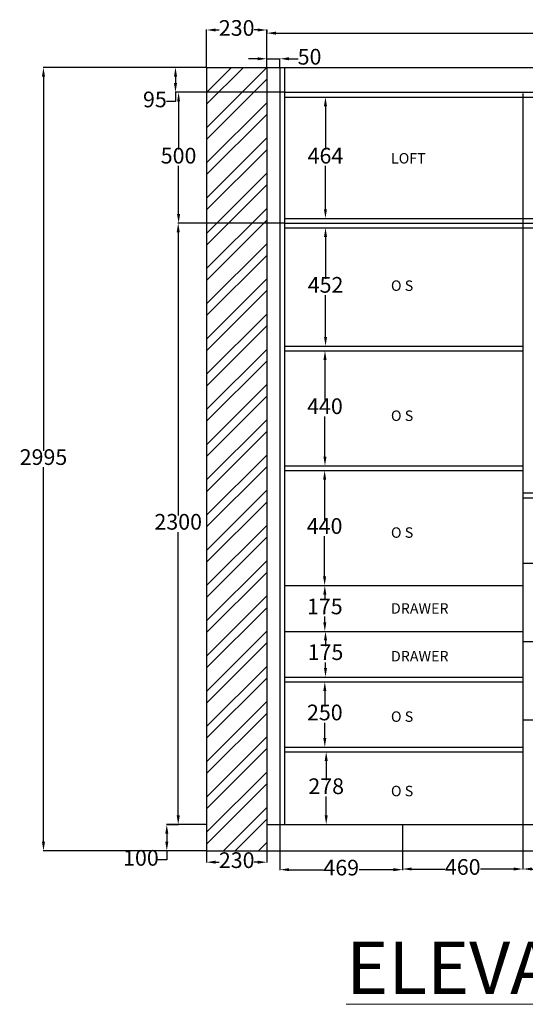
# Model space of a CAD drawing. Units: millimetres. Extents: x 1304 to 14372, y 283 to 7516.
# Tile 1 of 4: x 1304 to 3237, y 283 to 4048. Entities that reach past the tile are written whole.
import ezdxf

# ---------------------------------------------------------------- set-up
doc = ezdxf.new("R2010")
doc.units = ezdxf.units.MM
doc.layers.get('Defpoints').update_dxf_attribs({"color": 2})
for name, color, linetype, lineweight in [('A-ANNO-DIMS', 2, 'Continuous', 18), ('A-ANNO-TEXT', 3, 'Continuous', 18), ('A-FURN', 7, 'Continuous', 25), ('A-FURN-PATT', 8, 'Continuous', 13)]:
    doc.layers.add(name, color=color, linetype=linetype, lineweight=lineweight)
doc.styles.get("Standard").update_dxf_attribs({"font": 'arial.ttf'})
doc.dimstyles.new('ISO-25', dxfattribs={"dimtxt": 60, "dimasz": 35, "dimexe": 1.25, "dimexo": 0.625, "dimtad": 0, "dimtih": 1, "dimtoh": 1, "dimtxsty": 'Standard', "dimcen": 2.5, "dimclrd": 1, "dimclre": 3, "dimadec": 0, "dimazin": 0, "dimtfac": 1, "dimtmove": 0, "dimatfit": 3, "dimfxl": 1, "dimarcsym": 0})

# ---------------------------------------------------------------- blocks, each defined once
blk = doc.blocks.new('*D1')
at = {"layer": 'A-ANNO-DIMS', "color": 0, "lineweight": -2, "transparency": 16777216}
for p, q in [((2317.3, 3752.3), (2474.1, 3752.3)), ((2472.8, 3717.3), (2472.8, 3551.5)), ((2472.8, 3323.3), (2472.8, 3489)), ((2317.3, 3288.3), (2474.1, 3288.3))]:
    blk.add_line(p, q, dxfattribs=at)
at = {"layer": 'A-ANNO-DIMS', "color": 0, "transparency": 16777216}
for points in [[(2467, 3717.3), (2478.7, 3717.3), (2472.8, 3752.3)], [(2467, 3323.3), (2478.7, 3323.3), (2472.8, 3288.3)]]:
    blk.add_solid(points, dxfattribs=at)
at = {"layer": 'Defpoints', "color": 0, "transparency": 16777216}
for p in [(2316.6, 3752.3), (2316.6, 3288.3), (2472.8, 3288.3)]:
    blk.add_point(p, dxfattribs=at)
at = {"layer": 'A-ANNO-DIMS', "color": 0, "transparency": 16777216, "insert": (2472.8, 3520.3), "char_height": 60, "attachment_point": 5}
blk.add_mtext('464', dxfattribs=at)
blk = doc.blocks.new('*D2')
at = {"layer": 'A-ANNO-DIMS', "color": 0, "lineweight": -2, "transparency": 16777216}
for p, q in [((2317.3, 3252.3), (2474.4, 3252.3)), ((2473.2, 3217.3), (2473.2, 3057.5)), ((2473.2, 2835.3), (2473.2, 2995)), ((2317.3, 2800.3), (2474.4, 2800.3))]:
    blk.add_line(p, q, dxfattribs=at)
at = {"layer": 'A-ANNO-DIMS', "color": 0, "transparency": 16777216}
for points in [[(2467.4, 3217.3), (2479, 3217.3), (2473.2, 3252.3)], [(2467.4, 2835.3), (2479, 2835.3), (2473.2, 2800.3)]]:
    blk.add_solid(points, dxfattribs=at)
at = {"layer": 'Defpoints', "color": 0, "transparency": 16777216}
for p in [(2316.6, 3252.3), (2316.6, 2800.3), (2473.2, 2800.3)]:
    blk.add_point(p, dxfattribs=at)
at = {"layer": 'A-ANNO-DIMS', "color": 0, "transparency": 16777216, "insert": (2473.2, 3026.3), "char_height": 60, "attachment_point": 5}
blk.add_mtext('452', dxfattribs=at)
blk = doc.blocks.new('*D3')
at = {"layer": 'A-ANNO-DIMS', "color": 0, "lineweight": -2, "transparency": 16777216}
for p, q in [((2317.3, 2782.3), (2472.3, 2782.3)), ((2471, 2747.3), (2471, 2593.5)), ((2471, 2377.3), (2471, 2531)), ((2317.3, 2342.3), (2472.3, 2342.3))]:
    blk.add_line(p, q, dxfattribs=at)
at = {"layer": 'A-ANNO-DIMS', "color": 0, "transparency": 16777216}
for points in [[(2465.2, 2747.3), (2476.9, 2747.3), (2471, 2782.3)], [(2465.2, 2377.3), (2476.9, 2377.3), (2471, 2342.3)]]:
    blk.add_solid(points, dxfattribs=at)
at = {"layer": 'Defpoints', "color": 0, "transparency": 16777216}
for p in [(2316.6, 2782.3), (2316.6, 2342.3), (2471, 2342.3)]:
    blk.add_point(p, dxfattribs=at)
at = {"layer": 'A-ANNO-DIMS', "color": 0, "transparency": 16777216, "insert": (2471, 2562.3), "char_height": 60, "attachment_point": 5}
blk.add_mtext('440', dxfattribs=at)
blk = doc.blocks.new('*D4')
at = {"layer": 'A-ANNO-DIMS', "color": 0, "lineweight": -2, "transparency": 16777216}
for p, q in [((2317.3, 2324.3), (2470.9, 2324.3)), ((2469.7, 2289.3), (2469.7, 2135.5)), ((2469.7, 1919.3), (2469.7, 2073)), ((2317.3, 1884.3), (2470.9, 1884.3))]:
    blk.add_line(p, q, dxfattribs=at)
at = {"layer": 'A-ANNO-DIMS', "color": 0, "transparency": 16777216}
for points in [[(2463.8, 2289.3), (2475.5, 2289.3), (2469.7, 2324.3)], [(2463.8, 1919.3), (2475.5, 1919.3), (2469.7, 1884.3)]]:
    blk.add_solid(points, dxfattribs=at)
at = {"layer": 'Defpoints', "color": 0, "transparency": 16777216}
for p in [(2316.6, 2324.3), (2316.6, 1884.3), (2469.7, 1884.3)]:
    blk.add_point(p, dxfattribs=at)
at = {"layer": 'A-ANNO-DIMS', "color": 0, "transparency": 16777216, "insert": (2469.7, 2104.3), "char_height": 60, "attachment_point": 5}
blk.add_mtext('440', dxfattribs=at)
blk = doc.blocks.new('*D5')
at = {"layer": 'A-ANNO-DIMS', "color": 0, "lineweight": -2, "transparency": 16777216}
for p, q in [((2317.3, 1884.3), (2471.6, 1884.3)), ((2470.4, 1849.3), (2470.4, 1828)), ((2470.4, 1744.3), (2470.4, 1765.5)), ((2317.3, 1709.3), (2471.6, 1709.3))]:
    blk.add_line(p, q, dxfattribs=at)
at = {"layer": 'A-ANNO-DIMS', "color": 0, "transparency": 16777216}
for points in [[(2464.5, 1849.3), (2476.2, 1849.3), (2470.4, 1884.3)], [(2464.5, 1744.3), (2476.2, 1744.3), (2470.4, 1709.3)]]:
    blk.add_solid(points, dxfattribs=at)
at = {"layer": 'Defpoints', "color": 0, "transparency": 16777216}
for p in [(2316.6, 1884.3), (2316.6, 1709.3), (2470.4, 1709.3)]:
    blk.add_point(p, dxfattribs=at)
at = {"layer": 'A-ANNO-DIMS', "color": 0, "transparency": 16777216, "insert": (2470.4, 1796.8), "char_height": 60, "attachment_point": 5}
blk.add_mtext('175', dxfattribs=at)
blk = doc.blocks.new('*D6')
at = {"layer": 'A-ANNO-DIMS', "color": 0, "lineweight": -2, "transparency": 16777216}
for p, q in [((2317.3, 1709.3), (2474.3, 1709.3)), ((2473, 1674.3), (2473, 1653)), ((2473, 1569.3), (2473, 1590.5)), ((2317.3, 1534.3), (2474.3, 1534.3))]:
    blk.add_line(p, q, dxfattribs=at)
at = {"layer": 'A-ANNO-DIMS', "color": 0, "transparency": 16777216}
for points in [[(2467.2, 1674.3), (2478.8, 1674.3), (2473, 1709.3)], [(2467.2, 1569.3), (2478.8, 1569.3), (2473, 1534.3)]]:
    blk.add_solid(points, dxfattribs=at)
at = {"layer": 'Defpoints', "color": 0, "transparency": 16777216}
for p in [(2316.6, 1709.3), (2316.6, 1534.3), (2473, 1534.3)]:
    blk.add_point(p, dxfattribs=at)
at = {"layer": 'A-ANNO-DIMS', "color": 0, "transparency": 16777216, "insert": (2473, 1621.8), "char_height": 60, "attachment_point": 5}
blk.add_mtext('175', dxfattribs=at)
blk = doc.blocks.new('*D7')
at = {"layer": 'A-ANNO-DIMS', "color": 0, "lineweight": -2, "transparency": 16777216}
for p, q in [((2317.3, 1516.3), (2471.6, 1516.3)), ((2470.4, 1481.3), (2470.4, 1422.5)), ((2470.4, 1301.3), (2470.4, 1360)), ((2317.3, 1266.3), (2471.6, 1266.3))]:
    blk.add_line(p, q, dxfattribs=at)
at = {"layer": 'A-ANNO-DIMS', "color": 0, "transparency": 16777216}
for points in [[(2464.5, 1481.3), (2476.2, 1481.3), (2470.4, 1516.3)], [(2464.5, 1301.3), (2476.2, 1301.3), (2470.4, 1266.3)]]:
    blk.add_solid(points, dxfattribs=at)
at = {"layer": 'Defpoints', "color": 0, "transparency": 16777216}
for p in [(2316.6, 1516.3), (2316.6, 1266.3), (2470.4, 1266.3)]:
    blk.add_point(p, dxfattribs=at)
at = {"layer": 'A-ANNO-DIMS', "color": 0, "transparency": 16777216, "insert": (2470.4, 1391.3), "char_height": 60, "attachment_point": 5}
blk.add_mtext('250', dxfattribs=at)
blk = doc.blocks.new('*D8')
at = {"layer": 'A-ANNO-DIMS', "color": 0, "lineweight": -2, "transparency": 16777216}
for p, q in [((2317.3, 1248.3), (2476.9, 1248.3)), ((2475.7, 1213.3), (2475.7, 1140.5)), ((2475.7, 1005.3), (2475.7, 1078)), ((2317.3, 970.3), (2476.9, 970.3))]:
    blk.add_line(p, q, dxfattribs=at)
at = {"layer": 'A-ANNO-DIMS', "color": 0, "transparency": 16777216}
for points in [[(2469.8, 1213.3), (2481.5, 1213.3), (2475.7, 1248.3)], [(2469.8, 1005.3), (2481.5, 1005.3), (2475.7, 970.3)]]:
    blk.add_solid(points, dxfattribs=at)
at = {"layer": 'Defpoints', "color": 0, "transparency": 16777216}
for p in [(2316.6, 1248.3), (2316.6, 970.3), (2475.7, 970.3)]:
    blk.add_point(p, dxfattribs=at)
at = {"layer": 'A-ANNO-DIMS', "color": 0, "transparency": 16777216, "insert": (2475.7, 1109.3), "char_height": 60, "attachment_point": 5}
blk.add_mtext('278', dxfattribs=at)
blk = doc.blocks.new('*D9')
at = {"layer": 'A-ANNO-DIMS', "color": 0, "lineweight": -2, "transparency": 16777216}
for p, q in [((2018, 3865.3), (1393.8, 3865.3)), ((1395.1, 3830.3), (1395.1, 2399)), ((1395.1, 905.3), (1395.1, 2336.5)), ((2018, 870.3), (1393.8, 870.3))]:
    blk.add_line(p, q, dxfattribs=at)
at = {"layer": 'A-ANNO-DIMS', "color": 0, "transparency": 16777216}
for points in [[(1389.3, 3830.3), (1400.9, 3830.3), (1395.1, 3865.3)], [(1389.3, 905.3), (1400.9, 905.3), (1395.1, 870.3)]]:
    blk.add_solid(points, dxfattribs=at)
at = {"layer": 'Defpoints', "color": 0, "transparency": 16777216}
for p in [(2018.6, 3865.3), (1395.1, 870.3), (2018.6, 870.3)]:
    blk.add_point(p, dxfattribs=at)
at = {"layer": 'A-ANNO-DIMS', "color": 0, "transparency": 16777216, "insert": (1395.1, 2367.8), "char_height": 60, "attachment_point": 5}
blk.add_mtext('2995', dxfattribs=at)
blk = doc.blocks.new('*D10')
at = {"layer": 'A-ANNO-DIMS', "color": 0, "lineweight": -2, "transparency": 16777216}
for p, q in [((2018, 3865.3), (1898.5, 3865.3)), ((1899.7, 3830.3), (1899.7, 3805.3)), ((2018, 3770.3), (1898.5, 3770.3)), ((1899.7, 3770.3), (1899.7, 3735.3)), ((1899.7, 3735.3), (1864.7, 3735.3))]:
    blk.add_line(p, q, dxfattribs=at)
at = {"layer": 'A-ANNO-DIMS', "color": 0, "transparency": 16777216}
for points in [[(1893.9, 3830.3), (1905.6, 3830.3), (1899.7, 3865.3)], [(1893.9, 3805.3), (1905.6, 3805.3), (1899.7, 3770.3)]]:
    blk.add_solid(points, dxfattribs=at)
at = {"layer": 'Defpoints', "color": 0, "transparency": 16777216}
for p in [(2018.6, 3865.3), (1899.7, 3770.3), (2018.6, 3770.3)]:
    blk.add_point(p, dxfattribs=at)
at = {"layer": 'A-ANNO-DIMS', "color": 0, "transparency": 16777216, "insert": (1820.9, 3735.3), "char_height": 60, "attachment_point": 5}
blk.add_mtext('95', dxfattribs=at)
blk = doc.blocks.new('*D11')
at = {"layer": 'A-ANNO-DIMS', "color": 0, "lineweight": -2, "transparency": 16777216}
for p, q in [((2316, 3770.3), (1910.2, 3770.3)), ((1911.5, 3735.3), (1911.5, 3551.5)), ((1911.5, 3305.3), (1911.5, 3489)), ((2316, 3270.3), (1910.2, 3270.3))]:
    blk.add_line(p, q, dxfattribs=at)
at = {"layer": 'A-ANNO-DIMS', "color": 0, "transparency": 16777216}
for points in [[(1905.7, 3735.3), (1917.3, 3735.3), (1911.5, 3770.3)], [(1905.7, 3305.3), (1917.3, 3305.3), (1911.5, 3270.3)]]:
    blk.add_solid(points, dxfattribs=at)
at = {"layer": 'Defpoints', "color": 0, "transparency": 16777216}
for p in [(2316.6, 3770.3), (1911.5, 3270.3), (2316.6, 3270.3)]:
    blk.add_point(p, dxfattribs=at)
at = {"layer": 'A-ANNO-DIMS', "color": 0, "transparency": 16777216, "insert": (1911.5, 3520.3), "char_height": 60, "attachment_point": 5}
blk.add_mtext('500', dxfattribs=at)
blk = doc.blocks.new('*D12')
at = {"layer": 'A-ANNO-DIMS', "color": 0, "lineweight": -2, "transparency": 16777216}
for p, q in [((2018, 970.3), (1865.2, 970.3)), ((1866.4, 935.3), (1866.4, 905.3)), ((2018, 870.3), (1865.2, 870.3)), ((1866.4, 870.3), (1866.4, 835.3)), ((1866.4, 835.3), (1831.4, 835.3))]:
    blk.add_line(p, q, dxfattribs=at)
at = {"layer": 'A-ANNO-DIMS', "color": 0, "transparency": 16777216}
for points in [[(1860.6, 935.3), (1872.3, 935.3), (1866.4, 970.3)], [(1860.6, 905.3), (1872.3, 905.3), (1866.4, 870.3)]]:
    blk.add_solid(points, dxfattribs=at)
at = {"layer": 'Defpoints', "color": 0, "transparency": 16777216}
for p in [(2018.6, 970.3), (1866.4, 870.3), (2018.6, 870.3)]:
    blk.add_point(p, dxfattribs=at)
at = {"layer": 'A-ANNO-DIMS', "color": 0, "transparency": 16777216, "insert": (1767.5, 835.3), "char_height": 60, "attachment_point": 5}
blk.add_mtext('100', dxfattribs=at)
blk = doc.blocks.new('*D13')
at = {"layer": 'A-ANNO-DIMS', "color": 0, "lineweight": -2, "transparency": 16777216}
for p, q in [((1910.9, 3270.3), (1908.9, 3270.3)), ((1910.1, 3235.3), (1910.1, 2151.6)), ((1910.1, 1005.3), (1910.1, 2089)), ((1867.1, 970.3), (1911.4, 970.3))]:
    blk.add_line(p, q, dxfattribs=at)
at = {"layer": 'A-ANNO-DIMS', "color": 0, "transparency": 16777216}
for points in [[(1904.3, 3235.3), (1916, 3235.3), (1910.1, 3270.3)], [(1904.3, 1005.3), (1916, 1005.3), (1910.1, 970.3)]]:
    blk.add_solid(points, dxfattribs=at)
at = {"layer": 'Defpoints', "color": 0, "transparency": 16777216}
for p in [(1910.1, 3270.3), (1911.5, 3270.3), (1866.4, 970.3)]:
    blk.add_point(p, dxfattribs=at)
at = {"layer": 'A-ANNO-DIMS', "color": 0, "transparency": 16777216, "insert": (1910.1, 2120.3), "char_height": 60, "attachment_point": 5}
blk.add_mtext('2300', dxfattribs=at)
blk = doc.blocks.new('*D14')
at = {"layer": 'A-ANNO-DIMS', "color": 0, "lineweight": -2, "transparency": 16777216}
for p, q in [((2213.6, 3898.5), (2178.6, 3898.5)), ((2248.6, 3865.9), (2248.6, 3899.8)), ((2248.6, 3898.5), (2298.6, 3898.5)), ((2298.6, 3865.9), (2298.6, 3899.8)), ((2333.6, 3898.5), (2368.6, 3898.5))]:
    blk.add_line(p, q, dxfattribs=at)
at = {"layer": 'A-ANNO-DIMS', "color": 0, "transparency": 16777216}
for points in [[(2213.6, 3904.4), (2213.6, 3892.7), (2248.6, 3898.5)], [(2333.6, 3904.4), (2333.6, 3892.7), (2298.6, 3898.5)]]:
    blk.add_solid(points, dxfattribs=at)
at = {"layer": 'Defpoints', "color": 0, "transparency": 16777216}
for p in [(2298.6, 3898.5), (2248.6, 3865.3), (2298.6, 3865.3)]:
    blk.add_point(p, dxfattribs=at)
at = {"layer": 'A-ANNO-DIMS', "color": 0, "transparency": 16777216, "insert": (2412.1, 3898.5), "char_height": 60, "attachment_point": 5}
blk.add_mtext('50', dxfattribs=at)
blk = doc.blocks.new('*D15')
at = {"layer": 'A-ANNO-DIMS', "color": 0, "lineweight": -2, "transparency": 16777216}
for p, q in [((2018.6, 3865.9), (2018.6, 4009.9)), ((2053.6, 4008.6), (2066.3, 4008.6)), ((2213.6, 4008.6), (2201, 4008.6)), ((2248.6, 3865.9), (2248.6, 4009.9))]:
    blk.add_line(p, q, dxfattribs=at)
at = {"layer": 'A-ANNO-DIMS', "color": 0, "transparency": 16777216}
for points in [[(2053.6, 4014.4), (2053.6, 4002.8), (2018.6, 4008.6)], [(2213.6, 4014.4), (2213.6, 4002.8), (2248.6, 4008.6)]]:
    blk.add_solid(points, dxfattribs=at)
at = {"layer": 'Defpoints', "color": 0, "transparency": 16777216}
for p in [(2248.6, 4008.6), (2018.6, 3865.3), (2248.6, 3865.3)]:
    blk.add_point(p, dxfattribs=at)
at = {"layer": 'A-ANNO-DIMS', "color": 0, "transparency": 16777216, "insert": (2133.6, 4008.6), "char_height": 60, "attachment_point": 5}
blk.add_mtext('230', dxfattribs=at)
blk = doc.blocks.new('*D16')
at = {"layer": 'A-ANNO-DIMS', "color": 0, "lineweight": -2, "transparency": 16777216}
for p, q in [((2248.6, 4008), (2248.6, 3995.4)), ((2283.6, 3996.6), (4728.5, 3996.6)), ((7353.6, 3996.6), (4908.8, 3996.6)), ((7388.6, 3865.9), (7388.6, 3997.9))]:
    blk.add_line(p, q, dxfattribs=at)
at = {"layer": 'A-ANNO-DIMS', "color": 0, "transparency": 16777216}
for points in [[(2283.6, 4002.4), (2283.6, 3990.8), (2248.6, 3996.6)], [(7353.6, 4002.4), (7353.6, 3990.8), (7388.6, 3996.6)]]:
    blk.add_solid(points, dxfattribs=at)
at = {"layer": 'Defpoints', "color": 0, "transparency": 16777216}
for p in [(2248.6, 4008.6), (7388.6, 3996.6), (7388.6, 3865.3)]:
    blk.add_point(p, dxfattribs=at)
at = {"layer": 'A-ANNO-DIMS', "color": 0, "transparency": 16777216, "insert": (4818.6, 3996.6), "char_height": 60, "attachment_point": 5}
blk.add_mtext('5140', dxfattribs=at)
blk = doc.blocks.new('*D33')
at = {"layer": 'A-ANNO-DIMS', "color": 0, "lineweight": -2, "transparency": 16777216}
for p, q in [((2018.6, 869.7), (2018.6, 825.4)), ((2248.6, 869.7), (2248.6, 825.4)), ((2053.6, 826.6), (2066.3, 826.6)), ((2213.6, 826.6), (2201, 826.6))]:
    blk.add_line(p, q, dxfattribs=at)
at = {"layer": 'A-ANNO-DIMS', "color": 0, "transparency": 16777216}
for points in [[(2053.6, 832.4), (2053.6, 820.8), (2018.6, 826.6)], [(2213.6, 832.4), (2213.6, 820.8), (2248.6, 826.6)]]:
    blk.add_solid(points, dxfattribs=at)
at = {"layer": 'Defpoints', "color": 0, "transparency": 16777216}
for p in [(2018.6, 870.3), (2248.6, 870.3), (2248.6, 826.6)]:
    blk.add_point(p, dxfattribs=at)
at = {"layer": 'A-ANNO-DIMS', "color": 0, "transparency": 16777216, "insert": (2133.6, 826.6), "char_height": 60, "attachment_point": 5}
blk.add_mtext('230', dxfattribs=at)
blk = doc.blocks.new('*D34')
at = {"layer": 'A-ANNO-DIMS', "color": 0, "lineweight": -2, "transparency": 16777216}
for p, q in [((2298.6, 969.7), (2298.6, 796.7)), ((2767.6, 863.2), (2767.6, 796.7)), ((2333.6, 798), (2465, 798)), ((2732.6, 798), (2601.3, 798))]:
    blk.add_line(p, q, dxfattribs=at)
at = {"layer": 'A-ANNO-DIMS', "color": 0, "transparency": 16777216}
for points in [[(2333.6, 803.8), (2333.6, 792.2), (2298.6, 798)], [(2732.6, 803.8), (2732.6, 792.2), (2767.6, 798)]]:
    blk.add_solid(points, dxfattribs=at)
at = {"layer": 'Defpoints', "color": 0, "transparency": 16777216}
for p in [(2298.6, 970.3), (2767.6, 863.8), (2767.6, 798)]:
    blk.add_point(p, dxfattribs=at)
at = {"layer": 'A-ANNO-DIMS', "color": 0, "transparency": 16777216, "insert": (2533.1, 798), "char_height": 60, "attachment_point": 5}
blk.add_mtext('469', dxfattribs=at)
blk = doc.blocks.new('*D35')
at = {"layer": 'A-ANNO-DIMS', "color": 0, "lineweight": -2, "transparency": 16777216}
for p, q in [((2767.6, 969.7), (2767.6, 799.2)), ((3227.6, 969.7), (3227.6, 799.2)), ((2802.6, 800.5), (2929.6, 800.5)), ((3192.6, 800.5), (3065.7, 800.5))]:
    blk.add_line(p, q, dxfattribs=at)
at = {"layer": 'A-ANNO-DIMS', "color": 0, "transparency": 16777216}
for points in [[(2802.6, 806.3), (2802.6, 794.7), (2767.6, 800.5)], [(3192.6, 806.3), (3192.6, 794.7), (3227.6, 800.5)]]:
    blk.add_solid(points, dxfattribs=at)
at = {"layer": 'Defpoints', "color": 0, "transparency": 16777216}
for p in [(2767.6, 970.3), (3227.6, 970.3), (3227.6, 800.5)]:
    blk.add_point(p, dxfattribs=at)
at = {"layer": 'A-ANNO-DIMS', "color": 0, "transparency": 16777216, "insert": (2997.6, 800.5), "char_height": 60, "attachment_point": 5}
blk.add_mtext('460', dxfattribs=at)
blk = doc.blocks.new('*D36')
at = {"layer": 'A-ANNO-DIMS', "color": 0, "lineweight": -2, "transparency": 16777216}
for p, q in [((3227.6, 801.1), (3227.6, 801.7)), ((3262.6, 800.5), (3389.6, 800.5)), ((3652.6, 800.5), (3525.7, 800.5)), ((3687.6, 801.1), (3687.6, 801.7))]:
    blk.add_line(p, q, dxfattribs=at)
at = {"layer": 'A-ANNO-DIMS', "color": 0, "transparency": 16777216}
for points in [[(3262.6, 806.3), (3262.6, 794.7), (3227.6, 800.5)], [(3652.6, 806.3), (3652.6, 794.7), (3687.6, 800.5)]]:
    blk.add_solid(points, dxfattribs=at)
at = {"layer": 'Defpoints', "color": 0, "transparency": 16777216}
for p in [(3227.6, 800.5), (3687.6, 800.5), (3687.6, 800.5)]:
    blk.add_point(p, dxfattribs=at)
at = {"layer": 'A-ANNO-DIMS', "color": 0, "transparency": 16777216, "insert": (3457.6, 800.5), "char_height": 60, "attachment_point": 5}
blk.add_mtext('460', dxfattribs=at)

msp = doc.modelspace()

# ---------------------------------------------------------------- hatches: boundary and pattern name
at = {"layer": 'A-FURN-PATT'}
h = msp.add_hatch(dxfattribs=at)
h.set_pattern_fill('ANSI32', color=256, scale=10)
h.paths.add_polyline_path([(2018.643, 870.285), (2248.643, 870.285), (2248.643, 3865.285), (2018.643, 3865.285)])
h.paths.add_polyline_path([(7388.643, 870.285), (7618.643, 870.285), (7618.643, 3865.285), (7388.643, 3865.285)])

# ---------------------------------------------------------------- linework, layer by layer
at = {"layer": 'A-FURN'}
for p, q in [((2018.643, 3865.285), (2018.643, 870.285)), ((2018.643, 3865.285), (7618.643, 3865.285)), ((2248.643, 3865.285), (2248.643, 870.285)), ((2298.643, 3865.285), (2298.643, 970.285)), ((2316.643, 3865.285), (2316.643, 970.285)), ((2316.643, 3770.285), (7388.643, 3770.285)), ((3227.643, 3765.285), (3227.643, 970.285)), ((2316.643, 3752.285), (5067.643, 3752.285)), ((2316.643, 3288.285), (5067.643, 3288.285)), ((2316.643, 3270.285), (5545.643, 3270.285)), ((2316.643, 3252.285), (4165.643, 3252.285)), ((2316.643, 2800.285), (3227.643, 2800.285)), ((2316.643, 2782.285), (3227.643, 2782.285)), ((2316.643, 2342.285), (3227.643, 2342.285)), ((2316.643, 2324.285), (3227.643, 2324.285)), ((3227.643, 2238.285), (4147.643, 2238.285)), ((3227.643, 2220.285), (4147.643, 2220.285)), ((3227.643, 1970.285), (4147.643, 1970.285)), ((2316.643, 1884.285), (3227.643, 1884.285)), ((2316.643, 1709.285), (3227.643, 1709.285)), ((3227.643, 1670.285), (4147.643, 1670.285)), ((2316.643, 1534.285), (3227.643, 1534.285)), ((2316.643, 1516.285), (3227.643, 1516.285)), ((3227.643, 1370.285), (4147.643, 1370.285)), ((2316.643, 1266.285), (3227.643, 1266.285)), ((2316.643, 1248.285), (3227.643, 1248.285)), ((2248.643, 970.285), (3227.643, 970.285)), ((3227.643, 970.285), (4147.643, 970.285)), ((2018.643, 870.285), (7618.643, 870.285))]:
    msp.add_line(p, q, dxfattribs=at)

# ---------------------------------------------------------------- texts
at = {"layer": 'A-ANNO-TEXT', "attachment_point": 1}
for s, width, gutter_width, insert, char_height in [('LOFT', 605.86509, 50, (2723.167, 3538.046), 40), ('O S', 605.86509, 50, (2723.167, 3051.04), 40), ('O S', 605.86509, 50, (2723.167, 2553.744), 40), ('O S', 605.86509, 50, (2723.167, 2106.933), 40), ('DRAWER', 605.86509, 50, (2723.167, 1816.929), 40), ('DRAWER', 605.86509, 50, (2723.167, 1634.128), 40), ('O S', 605.86509, 50, (2723.167, 1403.233), 40), ('O S', 605.86509, 50, (2723.167, 1118.751), 40), ('{\\LELEVATION WITHOUT SHUTTER}', 5143.98189, 100, (2552.356, 523.2), 200)]:
    msp.add_mtext_dynamic_manual_height_columns(s, width=width, gutter_width=gutter_width, heights=[0], dxfattribs=dict(at, insert=insert, char_height=char_height))

# ---------------------------------------------------------------- dimensions: what is measured, and where the dimension line sits
at = {"layer": 'A-ANNO-DIMS'}
for base, p1, p2, picture, middle in [((2248.643, 4008.602), (2018.643, 3865.285), (2248.643, 3865.285), '*D15', (2133.643, 4008.602)), ((7388.643, 3996.603), (2248.643, 4008.602), (7388.643, 3865.285), '*D16', (4818.643, 3996.603)), ((2298.643, 3898.541), (2248.643, 3865.285), (2298.643, 3865.285), '*D14', (2412.139, 3898.541)), ((2767.643, 797.996), (2298.643, 970.285), (2767.643, 863.782), '*D34', (2533.143, 797.996)), ((3227.643, 800.49), (2767.643, 970.285), (3227.643, 970.285), '*D35', (2997.643, 800.49)), ((2248.643, 826.607), (2018.643, 870.285), (2248.643, 870.285), '*D33', (2133.643, 826.607)), ((3687.643, 800.49), (3227.643, 800.49), (3687.643, 800.49), '*D36', (3457.643, 800.49))]:
    dim = msp.add_linear_dim(base=base, p1=p1, p2=p2, dimstyle='ISO-25', override={"dimclrd": 0, "dimclre": 0, "dimclrt": 0}, dxfattribs=at)
    dim.commit()
    dim.dimension.update_dxf_attribs({"geometry": picture, "text_midpoint": middle})
for base, p1, p2, picture, middle in [((1395.095, 870.285), (2018.643, 3865.285), (2018.643, 870.285), '*D9', (1395.095, 2367.785)), ((1899.733, 3770.285), (2018.643, 3865.285), (2018.643, 3770.285), '*D10', (1820.909, 3735.285)), ((1911.484, 3270.285), (2316.643, 3770.285), (2316.643, 3270.285), '*D11', (1911.484, 3520.285)), ((2472.823, 3288.285), (2316.643, 3752.285), (2316.643, 3288.285), '*D1', (2472.823, 3520.285)), ((1910.133, 3270.285), (1866.44, 970.285), (1911.484, 3270.285), '*D13', (1910.133, 2120.285)), ((2473.195, 2800.285), (2316.643, 3252.285), (2316.643, 2800.285), '*D2', (2473.195, 3026.285)), ((2471.032, 2342.285), (2316.643, 2782.285), (2316.643, 2342.285), '*D3', (2471.032, 2562.285)), ((2469.668, 1884.285), (2316.643, 2324.285), (2316.643, 1884.285), '*D4', (2469.668, 2104.285)), ((2470.355, 1709.285), (2316.643, 1884.285), (2316.643, 1709.285), '*D5', (2470.355, 1796.785)), ((2473.011, 1534.285), (2316.643, 1709.285), (2316.643, 1534.285), '*D6', (2473.011, 1621.785)), ((2470.355, 1266.285), (2316.643, 1516.285), (2316.643, 1266.285), '*D7', (2470.355, 1391.285)), ((2475.666, 970.285), (2316.643, 1248.285), (2316.643, 970.285), '*D8', (2475.666, 1109.285)), ((1866.44, 870.285), (2018.643, 970.285), (2018.643, 870.285), '*D12', (1767.459, 835.285))]:
    dim = msp.add_linear_dim(base=base, p1=p1, p2=p2, angle=90, dimstyle='ISO-25', override={"dimclrd": 0, "dimclre": 0, "dimclrt": 0}, dxfattribs=at)
    dim.commit()
    dim.dimension.update_dxf_attribs({"geometry": picture, "text_midpoint": middle})

doc.saveas('drawing.dxf')
